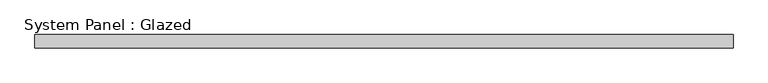
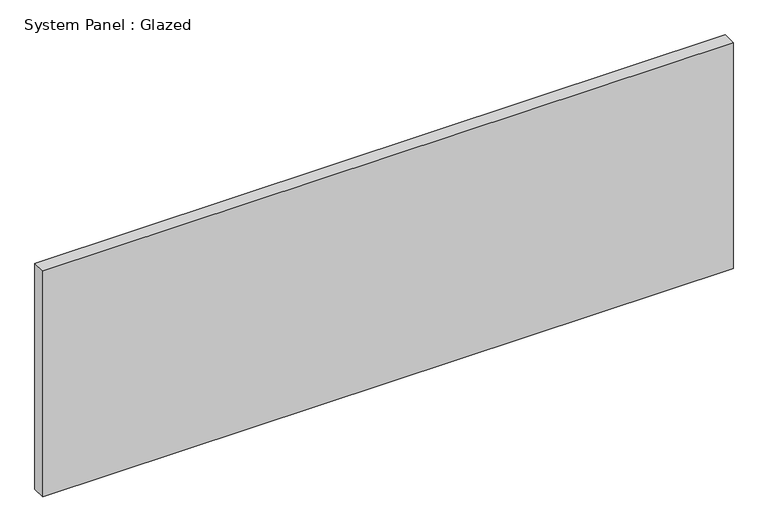
"""IFC4 building model written with IfcOpenShell, lengths in millimetres: plate geometry, System Panel : Glazed."""

from ifc_helpers import new_model, si_unit, origin, origin_with_axes, place, context, project, spatial, polyline, outline, extrude, source, transform, mapped, element, save


def system_panel_glazed_b1ae2562(model_context):
    return source(origin(), model_context, "Body", "SweptSolid", [
        extrude(outline(polyline([(654.0499999, 19.05), (-654.0499999, 19.05), (-654.0499999, 44.45), (654.0499999, 44.45), (654.0499999, 19.05)])), origin_with_axes(), (0.0, 0.0, 1.0), 452.9666667),
    ])


if __name__ == "__main__":
    model = new_model("IFC4")
    model_context = context("Model", 3, world=origin())
    ifc_project = project(units=[si_unit("LENGTHUNIT", "METRE", prefix="MILLI")], contexts=[model_context])
    site = spatial("IfcSite", under=ifc_project)
    building = spatial("IfcBuilding", under=site)
    placement = place(None, origin())
    system_panel_glazed_shape = system_panel_glazed_b1ae2562(model_context)
    element("IfcPlate", 1, ObjectType="System Panel : Glazed", at=placement, inside=building, context=model_context, shape_type="MappedRepresentation", body=[
        mapped(system_panel_glazed_shape, transform((0.0, 0.0, 0.0), x_axis=(1.0, 0.0, 0.0), y_axis=(0.0, 1.0, 0.0), z_axis=(0.0, 0.0, 1.0))),
    ])
    save(model, "model.ifc")

# Revit data of these elements
# Type "System Panel : Glazed"
#   Construction Type Id = "GSP4R"
#   Analytic Construction = "1/8 in Pilkington single glazing"
#   Visual Light Transmittance = 0.9
#   Solar Heat Gain Coefficient = 0.86
#   Heat Transfer Coefficient (U) = 1.18115 BTU/(h·ft²·°F)
#   Define Thermal Properties by = 1
# Element 1 (IfcPlate, "System Panel : Glazed")
#   Materials on its faces: "glass panel 223"
# Materials
#   "glass panel 223": class "Generic", colour RGB 120 120 120, transparency 0, Cost = 0
